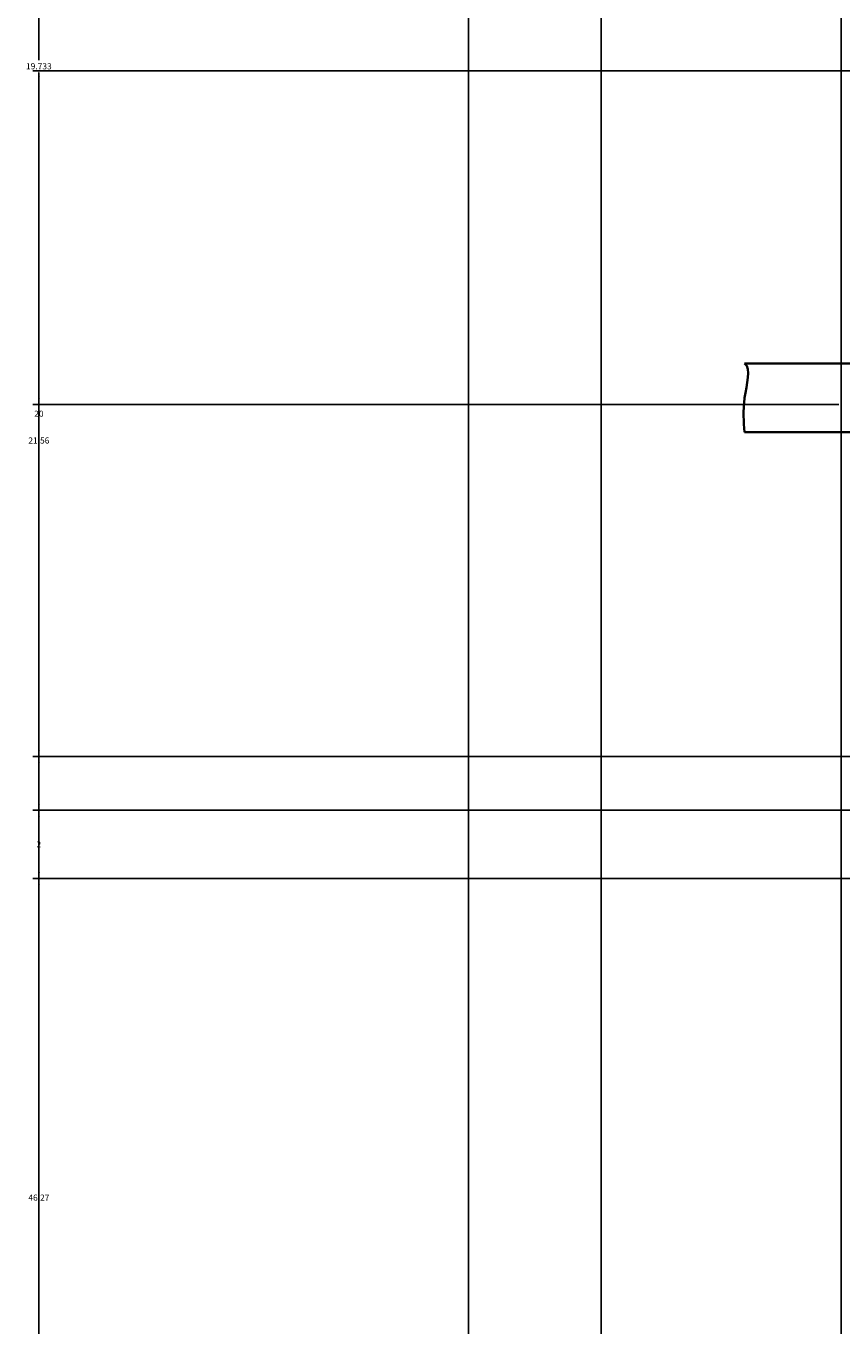
# Model space of a CAD drawing. Units: inches. Extents: x 2812 to 3051, y 1398 to 1659.
# Tile 4 of 65: x 2812 to 2835, y 1435 to 1473. Entities that reach past the tile are written whole.
import ezdxf

# ---------------------------------------------------------------- set-up
doc = ezdxf.new("R2010")
doc.units = ezdxf.units.IN
doc.layers.add('A-ANNO-DIMS', color=2, linetype='Continuous', lineweight=18)
doc.layers.add('P-SANR-PIPE', color=4, linetype='Continuous', lineweight=35)
doc.styles.get("Standard").update_dxf_attribs({"font": 'arial.ttf'})
doc.dimstyles.get("Standard").update_dxf_attribs({"dimtxt": 0.18, "dimasz": 0.18, "dimexe": 0.18, "dimexo": 0.0625, "dimgap": 0.09, "dimtad": 0, "dimtih": 1, "dimtoh": 1, "dimdec": 4, "dimzin": 0, "dimdsep": 46, "dimtxsty": 'Standard', "dimcen": 0.09, "dimadec": 0, "dimazin": 0, "dimtfac": 1, "dimtdec": 4, "dimtofl": 0, "dimtmove": 0, "dimatfit": 3, "dimfxl": 1, "dimtolj": 1, "dimtzin": 0, "dimarcsym": 0})

# ---------------------------------------------------------------- blocks, each defined once
blk = doc.blocks.new('PIPE-TEE-SECTION')
for p, q in [((1.921, 13.381), (0, 13.381)), ((0, 13.381), (0, 12.795)), ((1.921, 12.795), (1.921, 13.381)), ((0, 12.795), (0, 10.254)), ((1.921, 12.235), (1.921, 12.795)), ((2.641, 12.254), (1.921, 12.254)), ((1.921, 10.254), (1.921, 12.235)), ((2.299, 12.254), (2.299, 10.254)), ((2.641, 10.254), (2.641, 12.254)), ((2.641, 12.254), (14.641, 12.254)), ((2.641, 12.254), (3.141, 12.254)), ((3.141, 12.254), (3.141, 10.254)), ((0, 10.254), (1.921, 10.254)), ((0, 10.254), (0, 0)), ((2.299, 10.254), (1.921, 10.254)), ((1.921, 10.254), (1.921, 9.254)), ((14.641, 10.254), (2.299, 10.254)), ((0, 9.254), (1.921, 9.254)), ((0, 9), (0, 9.254)), ((1.921, 9.254), (1.921, 9)), ((1.921, 9), (0, 9)), ((1.921, 9), (1.921, 0)), ((1.921, 0), (0, 0))]:
    blk.add_line(p, q)
blk.add_open_spline([(14.641, 10.254), (14.669, 10.56), (14.725, 11.17), (14.444, 12.118), (14.641, 12.254)], degree=3)
blk = doc.blocks.new('*D27')
at = {"layer": 'A-ANNO-DIMS', "color": 0, "lineweight": -2, "transparency": 16777216}
for p, q in [((2824.521, 1594.167), (2824.521, 1397.505)), ((2835.385, 1550.757), (2835.385, 1397.505)), ((2824.701, 1397.685), (2829.498, 1397.685)), ((2835.205, 1397.685), (2830.408, 1397.685))]:
    blk.add_line(p, q, dxfattribs=at)
at = {"layer": 'A-ANNO-DIMS', "color": 0, "transparency": 16777216}
for points in [[(2824.701, 1397.715), (2824.701, 1397.655), (2824.521, 1397.685)], [(2835.205, 1397.715), (2835.205, 1397.655), (2835.385, 1397.685)]]:
    blk.add_solid(points, dxfattribs=at)
at = {"layer": 'Defpoints', "color": 0, "transparency": 16777216}
for p in [(2824.521, 1594.23), (2835.385, 1550.82), (2835.385, 1397.685)]:
    blk.add_point(p, dxfattribs=at)
at = {"layer": 'A-ANNO-DIMS', "color": 0, "transparency": 16777216, "insert": (2829.953, 1397.685), "char_height": 0.18, "attachment_point": 5}
blk.add_mtext('\\A1;10.863', dxfattribs=at)
blk = doc.blocks.new('*D41')
at = {"layer": 'A-ANNO-DIMS', "color": 0, "lineweight": -2, "transparency": 16777216}
for p, q in [((2828.385, 1489.973), (2828.385, 1397.505)), ((2826.385, 1409.973), (2826.385, 1397.505)), ((2826.565, 1397.685), (2827.235, 1397.685)), ((2828.205, 1397.685), (2827.535, 1397.685))]:
    blk.add_line(p, q, dxfattribs=at)
at = {"layer": 'A-ANNO-DIMS', "color": 0, "transparency": 16777216}
for points in [[(2826.565, 1397.715), (2826.565, 1397.655), (2826.385, 1397.685)], [(2828.205, 1397.715), (2828.205, 1397.655), (2828.385, 1397.685)]]:
    blk.add_solid(points, dxfattribs=at)
at = {"layer": 'Defpoints', "color": 0, "transparency": 16777216}
for p in [(2828.385, 1490.035), (2826.385, 1410.035), (2828.385, 1397.685)]:
    blk.add_point(p, dxfattribs=at)
at = {"layer": 'A-ANNO-DIMS', "color": 0, "transparency": 16777216, "insert": (2827.385, 1397.685), "char_height": 0.18, "attachment_point": 5}
blk.add_mtext('\\A1;2', dxfattribs=at)
blk = doc.blocks.new('*D42')
at = {"layer": 'A-ANNO-DIMS', "color": 0, "lineweight": -2, "transparency": 16777216}
for p, q in [((2828.385, 1489.973), (2828.385, 1397.505)), ((2847.686, 1487.973), (2847.686, 1397.505)), ((2828.565, 1397.685), (2837.72, 1397.685)), ((2847.506, 1397.685), (2838.351, 1397.685))]:
    blk.add_line(p, q, dxfattribs=at)
at = {"layer": 'A-ANNO-DIMS', "color": 0, "transparency": 16777216}
for points in [[(2828.565, 1397.715), (2828.565, 1397.655), (2828.385, 1397.685)], [(2847.506, 1397.715), (2847.506, 1397.655), (2847.686, 1397.685)]]:
    blk.add_solid(points, dxfattribs=at)
at = {"layer": 'Defpoints', "color": 0, "transparency": 16777216}
for p in [(2828.385, 1490.035), (2847.686, 1488.035), (2847.686, 1397.685)]:
    blk.add_point(p, dxfattribs=at)
at = {"layer": 'A-ANNO-DIMS', "color": 0, "transparency": 16777216, "insert": (2838.036, 1397.685), "char_height": 0.18, "attachment_point": 5}
blk.add_mtext('\\A1;19.3', dxfattribs=at)
blk = doc.blocks.new('*D50')
at = {"layer": 'A-ANNO-DIMS', "color": 0, "lineweight": -2, "transparency": 16777216}
for p, q in [((2835.322, 1462.303), (2811.806, 1462.303)), ((2811.986, 1462.123), (2811.986, 1439.351)), ((2811.986, 1416.215), (2811.986, 1438.987)), ((2835.322, 1416.035), (2811.806, 1416.035))]:
    blk.add_line(p, q, dxfattribs=at)
at = {"layer": 'A-ANNO-DIMS', "color": 0, "transparency": 16777216}
for points in [[(2811.956, 1462.123), (2812.016, 1462.123), (2811.986, 1462.303)], [(2811.956, 1416.215), (2812.016, 1416.215), (2811.986, 1416.035)]]:
    blk.add_solid(points, dxfattribs=at)
at = {"layer": 'Defpoints', "color": 0, "transparency": 16777216}
for p in [(2811.986, 1462.303), (2835.385, 1462.303), (2835.385, 1416.035)]:
    blk.add_point(p, dxfattribs=at)
at = {"layer": 'A-ANNO-DIMS', "color": 0, "transparency": 16777216, "insert": (2811.986, 1439.169), "char_height": 0.18, "attachment_point": 5}
blk.add_mtext('\\A1;46.27', dxfattribs=at)
blk = doc.blocks.new('*D51')
at = {"layer": 'A-ANNO-DIMS', "color": 0, "lineweight": -2, "transparency": 16777216}
for p, q in [((2835.322, 1482.035), (2811.806, 1482.035)), ((2811.986, 1481.855), (2811.986, 1472.351)), ((2811.986, 1462.483), (2811.986, 1471.987)), ((2835.322, 1462.303), (2811.806, 1462.303))]:
    blk.add_line(p, q, dxfattribs=at)
at = {"layer": 'A-ANNO-DIMS', "color": 0, "transparency": 16777216}
for points in [[(2811.956, 1481.855), (2812.016, 1481.855), (2811.986, 1482.035)], [(2811.956, 1462.483), (2812.016, 1462.483), (2811.986, 1462.303)]]:
    blk.add_solid(points, dxfattribs=at)
at = {"layer": 'Defpoints', "color": 0, "transparency": 16777216}
for p in [(2811.986, 1482.035), (2835.385, 1482.035), (2835.385, 1462.303)]:
    blk.add_point(p, dxfattribs=at)
at = {"layer": 'A-ANNO-DIMS', "color": 0, "transparency": 16777216, "insert": (2811.986, 1472.169), "char_height": 0.18, "attachment_point": 5}
blk.add_mtext('\\A1;19.733', dxfattribs=at)
blk = doc.blocks.new('*D56')
at = {"layer": 'A-ANNO-DIMS', "color": 0, "lineweight": -2, "transparency": 16777216}
for p, q in [((2880.322, 1452.035), (2811.806, 1452.035)), ((2811.986, 1451.855), (2811.986, 1434.217)), ((2811.986, 1416.215), (2811.986, 1433.853)), ((2952.322, 1416.035), (2811.806, 1416.035))]:
    blk.add_line(p, q, dxfattribs=at)
at = {"layer": 'A-ANNO-DIMS', "color": 0, "transparency": 16777216}
for points in [[(2811.956, 1451.855), (2812.016, 1451.855), (2811.986, 1452.035)], [(2811.956, 1416.215), (2812.016, 1416.215), (2811.986, 1416.035)]]:
    blk.add_solid(points, dxfattribs=at)
at = {"layer": 'Defpoints', "color": 0, "transparency": 16777216}
for p in [(2811.986, 1452.035), (2880.385, 1452.035), (2952.385, 1416.035)]:
    blk.add_point(p, dxfattribs=at)
at = {"layer": 'A-ANNO-DIMS', "color": 0, "transparency": 16777216, "insert": (2811.986, 1434.035), "char_height": 0.18, "attachment_point": 5}
blk.add_mtext('\\A1;36', dxfattribs=at)
blk = doc.blocks.new('*D57')
at = {"layer": 'A-ANNO-DIMS', "color": 0, "lineweight": -2, "transparency": 16777216}
for p, q in [((2880.322, 1472.035), (2811.806, 1472.035)), ((2811.986, 1471.855), (2811.986, 1462.217)), ((2811.986, 1452.215), (2811.986, 1461.853)), ((2880.322, 1452.035), (2811.806, 1452.035))]:
    blk.add_line(p, q, dxfattribs=at)
at = {"layer": 'A-ANNO-DIMS', "color": 0, "transparency": 16777216}
for points in [[(2811.956, 1471.855), (2812.016, 1471.855), (2811.986, 1472.035)], [(2811.956, 1452.215), (2812.016, 1452.215), (2811.986, 1452.035)]]:
    blk.add_solid(points, dxfattribs=at)
at = {"layer": 'Defpoints', "color": 0, "transparency": 16777216}
for p in [(2811.986, 1472.035), (2880.385, 1472.035), (2880.385, 1452.035)]:
    blk.add_point(p, dxfattribs=at)
at = {"layer": 'A-ANNO-DIMS', "color": 0, "transparency": 16777216, "insert": (2811.986, 1462.035), "char_height": 0.18, "attachment_point": 5}
blk.add_mtext('\\A1;20', dxfattribs=at)
blk = doc.blocks.new('*D75')
at = {"layer": 'A-ANNO-DIMS', "color": 0, "lineweight": -2, "transparency": 16777216}
for p, q in [((2963.812, 1448.474), (2811.806, 1448.474)), ((2811.986, 1448.294), (2811.986, 1432.437)), ((2811.986, 1416.215), (2811.986, 1432.073)), ((2961.322, 1416.035), (2811.806, 1416.035))]:
    blk.add_line(p, q, dxfattribs=at)
at = {"layer": 'A-ANNO-DIMS', "color": 0, "transparency": 16777216}
for points in [[(2811.956, 1448.294), (2812.016, 1448.294), (2811.986, 1448.474)], [(2811.956, 1416.215), (2812.016, 1416.215), (2811.986, 1416.035)]]:
    blk.add_solid(points, dxfattribs=at)
at = {"layer": 'Defpoints', "color": 0, "transparency": 16777216}
for p in [(2811.986, 1448.474), (2963.874, 1448.474), (2961.385, 1416.035)]:
    blk.add_point(p, dxfattribs=at)
at = {"layer": 'A-ANNO-DIMS', "color": 0, "transparency": 16777216, "insert": (2811.986, 1432.255), "char_height": 0.18, "attachment_point": 5}
blk.add_mtext('\\A1;32.44', dxfattribs=at)
blk = doc.blocks.new('*D76')
at = {"layer": 'A-ANNO-DIMS', "color": 0, "lineweight": -2, "transparency": 16777216}
for p, q in [((2963.812, 1450.474), (2811.806, 1450.474)), ((2811.986, 1450.294), (2811.986, 1449.654)), ((2811.986, 1448.654), (2811.986, 1449.293)), ((2963.812, 1448.474), (2811.806, 1448.474))]:
    blk.add_line(p, q, dxfattribs=at)
at = {"layer": 'A-ANNO-DIMS', "color": 0, "transparency": 16777216}
for points in [[(2811.956, 1450.294), (2812.016, 1450.294), (2811.986, 1450.474)], [(2811.956, 1448.654), (2812.016, 1448.654), (2811.986, 1448.474)]]:
    blk.add_solid(points, dxfattribs=at)
at = {"layer": 'Defpoints', "color": 0, "transparency": 16777216}
for p in [(2811.986, 1450.474), (2963.874, 1450.474), (2963.874, 1448.474)]:
    blk.add_point(p, dxfattribs=at)
at = {"layer": 'A-ANNO-DIMS', "color": 0, "transparency": 16777216, "insert": (2811.986, 1449.474), "char_height": 0.18, "attachment_point": 5}
blk.add_mtext('\\A1;2', dxfattribs=at)
blk = doc.blocks.new('*D77')
at = {"layer": 'A-ANNO-DIMS', "color": 0, "lineweight": -2, "transparency": 16777216}
for p, q in [((2961.322, 1472.035), (2811.806, 1472.035)), ((2811.986, 1471.855), (2811.986, 1461.436)), ((2811.986, 1450.654), (2811.986, 1461.073)), ((2963.812, 1450.474), (2811.806, 1450.474))]:
    blk.add_line(p, q, dxfattribs=at)
at = {"layer": 'A-ANNO-DIMS', "color": 0, "transparency": 16777216}
for points in [[(2811.956, 1471.855), (2812.016, 1471.855), (2811.986, 1472.035)], [(2811.956, 1450.654), (2812.016, 1450.654), (2811.986, 1450.474)]]:
    blk.add_solid(points, dxfattribs=at)
at = {"layer": 'Defpoints', "color": 0, "transparency": 16777216}
for p in [(2811.986, 1472.035), (2961.385, 1472.035), (2963.874, 1450.474)]:
    blk.add_point(p, dxfattribs=at)
at = {"layer": 'A-ANNO-DIMS', "color": 0, "transparency": 16777216, "insert": (2811.986, 1461.255), "char_height": 0.18, "attachment_point": 5}
blk.add_mtext('\\A1;21.56', dxfattribs=at)

msp = doc.modelspace()

# ---------------------------------------------------------------- block references
at = {"layer": 'P-SANR-PIPE', "extrusion": (0, 0, -1), "zscale": -1}
msp.add_blockref('PIPE-TEE-SECTION', (-2847.2154, 1451.2415), dxfattribs=at)

# ---------------------------------------------------------------- dimensions: what is measured, and where the dimension line sits
at = {"layer": 'A-ANNO-DIMS'}
for base, p1, p2, override, picture, middle in [((2835.384907, 1397.685398), (2824.521409, 1594.229631), (2835.384907, 1550.819971), {"dimdec": 3, "dimlfac": 1, "dimrnd": 0, "dimzin": 0, "dimdsep": 46, "dimlunit": 2}, '*D27', (2829.953158, 1397.685398)), ((2828.3849, 1397.6854), (2826.3849, 1410.0354), (2828.3849, 1490.0354), {"dimdec": 0, "dimlfac": 1, "dimrnd": 0, "dimzin": 0, "dimdsep": 46, "dimlunit": 2}, '*D41', (2827.3849, 1397.6854)), ((2847.6863, 1397.6854), (2828.3849, 1490.0354), (2847.6863, 1488.0354), {"dimdec": 1, "dimlfac": 1, "dimrnd": 0, "dimzin": 0, "dimdsep": 46, "dimlunit": 2}, '*D42', (2838.0356, 1397.6854))]:
    dim = msp.add_linear_dim(base=base, p1=p1, p2=p2, dimstyle='Standard', override=override, dxfattribs=at)
    dim.commit()
    dim.dimension.update_dxf_attribs({"geometry": picture, "text_midpoint": middle})
for base, p1, p2, override, picture, middle in [((2811.9855, 1482.0354), (2835.3849, 1462.3026), (2835.3849, 1482.0354), {"dimdec": 3, "dimlfac": 1, "dimrnd": 0, "dimzin": 0, "dimdsep": 46, "dimlunit": 2}, '*D51', (2811.9855, 1472.169)), ((2811.9855, 1472.0354), (2963.8741, 1450.4738), (2961.3849, 1472.0354), {"dimdec": 2, "dimlfac": 1, "dimrnd": 0, "dimzin": 0, "dimdsep": 46, "dimlunit": 2}, '*D77', (2811.9855, 1461.2546)), ((2811.9855, 1472.0354), (2880.3849, 1452.0354), (2880.3849, 1472.0354), {"dimdec": 0, "dimlfac": 1, "dimrnd": 0, "dimzin": 0, "dimdsep": 46, "dimlunit": 2}, '*D57', (2811.9855, 1462.0354)), ((2811.9855, 1462.3026), (2835.3849, 1416.0354), (2835.3849, 1462.3026), {"dimdec": 2, "dimlfac": 1, "dimrnd": 0, "dimzin": 0, "dimdsep": 46, "dimlunit": 2}, '*D50', (2811.9855, 1439.169)), ((2811.9855, 1452.0354), (2952.3849, 1416.0354), (2880.3849, 1452.0354), {"dimdec": 0, "dimlfac": 1, "dimrnd": 0, "dimzin": 0, "dimdsep": 46, "dimlunit": 2}, '*D56', (2811.9855, 1434.0354)), ((2811.9855, 1450.4738), (2963.8741, 1448.4738), (2963.8741, 1450.4738), {"dimdec": 0, "dimlfac": 1, "dimrnd": 0, "dimzin": 0, "dimdsep": 46, "dimlunit": 2}, '*D76', (2811.9855, 1449.4738)), ((2811.9855, 1448.4738), (2961.3849, 1416.0354), (2963.8741, 1448.4738), {"dimdec": 2, "dimlfac": 1, "dimrnd": 0, "dimzin": 0, "dimdsep": 46, "dimlunit": 2}, '*D75', (2811.9855, 1432.2546))]:
    dim = msp.add_linear_dim(base=base, p1=p1, p2=p2, angle=90, dimstyle='Standard', override=override, dxfattribs=at)
    dim.commit()
    dim.dimension.update_dxf_attribs({"geometry": picture, "text_midpoint": middle})

doc.saveas('drawing.dxf')
